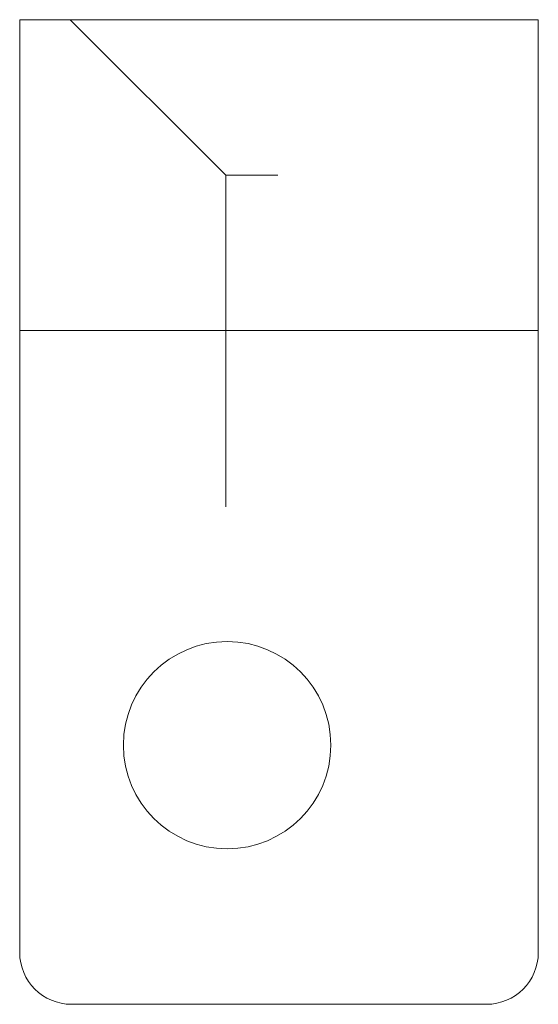
# Model space of a CAD drawing. Units: millimetres. Extents: x 201.3 to 251.3, y 605.6 to 700.6.
import ezdxf

# ---------------------------------------------------------------- set-up
doc = ezdxf.new("R2010")
doc.units = ezdxf.units.MM
doc.layers.add('M-CONS', color=8, linetype='Continuous', lineweight=18)

msp = doc.modelspace()

# ---------------------------------------------------------------- linework, layer by layer
at = {"layer": 'M-CONS'}
for p, q in [((201.312, 670.629, -57), (201.312, 700.629, -57)), ((201.312, 700.629, -57), (251.312, 700.629, -57)), ((201.312, 700.629, -49), (251.312, 700.629, -49)), ((201.312, 610.629, -49), (201.312, 700.629, -49)), ((201.312, 700.629, -57), (251.312, 700.629, -57)), ((201.312, 700.629, -57), (201.312, 670.629, -57)), ((201.312, 700.629, -49), (201.312, 685.629, -49)), ((251.312, 700.629), (251.312, 700.629, -65)), ((251.312, 700.629, -65), (251.312, 670.629, -65)), ((251.312, 670.629, -57), (251.312, 700.629, -57)), ((251.312, 700.629, -49), (251.312, 610.629, -49)), ((201.312, 610.629, -57), (201.312, 670.629, -57)), ((201.312, 670.629, -57), (251.312, 670.629, -57)), ((251.312, 670.629, -65), (251.312, 670.629, -57)), ((251.312, 670.629, -57), (251.312, 610.629, -57)), ((246.312, 605.629, -57), (206.312, 605.629, -57)), ((246.312, 605.629, -49), (206.312, 605.629, -49))]:
    msp.add_line(p, q, dxfattribs=at)
at = {"layer": 'M-CONS', "extrusion": (-1, 0, 0)}
for p, q in [((201.312, 610.629, -49), (201.312, 700.629, -49)), ((201.312, 700.629, -49), (201.312, 700.629, -57)), ((201.312, 700.629, -57), (201.312, 610.629, -57))]:
    msp.add_line(p, q, dxfattribs=at)
at = {"layer": 'M-CONS', "extrusion": (0, 0, -1)}
for p, q in [((201.312, 700.629, -57), (201.312, 610.629, -57)), ((251.312, 700.629, -57), (201.312, 700.629, -57)), ((251.312, 610.629, -57), (251.312, 700.629, -57)), ((206.312, 605.629, -57), (246.312, 605.629, -57))]:
    msp.add_line(p, q, dxfattribs=at)
at = {"layer": 'M-CONS', "extrusion": (0, 1, 0)}
for p, q in [((201.312, 700.629, -65), (201.312, 700.629, -57)), ((201.312, 700.629, -57), (251.312, 700.629, -57)), ((201.312, 700.629, -65), (251.312, 700.629, -65)), ((251.312, 700.629, -65), (251.312, 700.629, -57))]:
    msp.add_line(p, q, dxfattribs=at)
at = {"layer": 'M-CONS', "extrusion": (0, -1, 0)}
for p, q in [((221.189, 685.629, -15), (206.189, 700.629, -65)), ((226.189, 685.629, -15), (221.189, 685.629, -15)), ((221.189, 685.629, -15), (226.189, 685.629, -15)), ((246.312, 605.629, -49), (206.312, 605.629, -49)), ((206.312, 605.629, -57), (246.312, 605.629, -57))]:
    msp.add_line(p, q, dxfattribs=at)
at = {"layer": 'M-CONS', "extrusion": (1, 0, 0)}
for p, q in [((251.312, 700.629, -49), (251.312, 700.629, -57)), ((251.312, 700.629, -49), (251.312, 610.629, -49)), ((251.312, 610.629, -57), (251.312, 700.629, -57))]:
    msp.add_line(p, q, dxfattribs=at)
at = {"layer": 'M-CONS', "elevation": -57}
msp.add_lwpolyline([(201.312, 670.629), (201.312, 670.629), (201.312, 670.629), (201.312, 670.629)], close=True, dxfattribs=at)
at = {"layer": 'M-CONS'}
msp.add_polyline3d([(221.189, 653.629, -49), (221.189, 685.629, -15), (221.189, 685.629, -49)], close=True, dxfattribs=at)
msp.add_circle((221.312, 630.629, -49), 10, dxfattribs=at)
for centre, start, end in [((206.312, 610.629, -57), 180, 270), ((206.312, 610.629, -49), 180, 270), ((246.312, 610.629, -57), 270, 0), ((246.312, 610.629, -49), 270, 0)]:
    msp.add_arc(centre, 5, start, end, dxfattribs=at)

doc.saveas('drawing.dxf')
